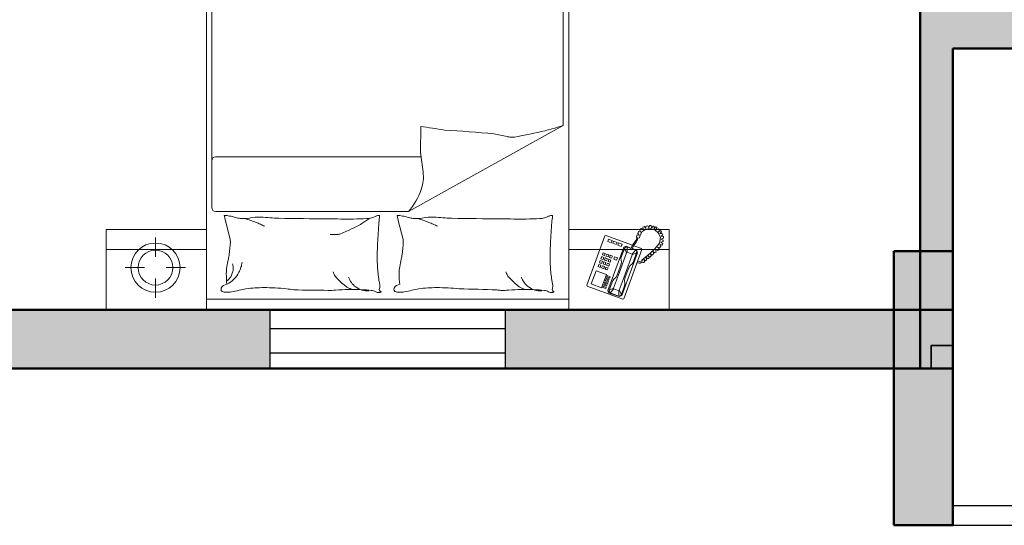
# Model space of a CAD drawing. Units: inches. Extents: x -7 to 1228, y -146 to 1091.
# Tile 21 of 88: x 664 to 815, y 36 to 113. Entities that reach past the tile are written whole.
import ezdxf

# ---------------------------------------------------------------- set-up
doc = ezdxf.new("R2010")
doc.units = ezdxf.units.IN
for name, color, linetype, lineweight in [('A-COLS', 6, 'Continuous', 35), ('A-FURN', 8, 'Continuous', 18), ('A-GLAZ', 175, 'Continuous', 25), ('A-WALL', 7, 'Continuous', 50), ('A-WALL-PATT', 251, 'Continuous', 13)]:
    doc.layers.add(name, color=color, linetype=linetype, lineweight=lineweight)
doc.styles.add('DIM_FONT', font='SIMPLEX.shx', dxfattribs={"width": 0.8})

# ---------------------------------------------------------------- blocks, each defined once
blk = doc.blocks.new('A$C4F634EDD')
for p, q in [((0, 2.6295), (0, 2.2295)), ((0.5, 2.6295), (0, 2.6295)), ((0.5, 2.6295), (2.3, 2.6295)), ((0.5, 0.5295), (0.5, 2.6295)), ((0.5, 2.2295), (0.5, 2.6295)), ((2.3, 2.6295), (2.3, 0.5295)), ((2.3, 2.6295), (2.8, 2.6295)), ((2.3, 2.2295), (2.3, 2.6295)), ((2.8, 2.6295), (2.8, 2.2295)), ((0.2457, 2.5697), (0.2457, 2.4733)), ((0.5, 2.5771), (2.3, 2.5771)), ((2.392, 2.5115), (2.5692, 2.5765)), ((2.4985, 2.5445), (2.5516, 2.564)), ((2.5062, 2.5454), (2.5004, 2.5392)), ((2.5062, 2.5454), (2.5487, 2.561)), ((2.5235, 2.5256), (2.5062, 2.5454)), ((2.5483, 2.5347), (2.5487, 2.561)), ((2.5487, 2.561), (2.5571, 2.56)), ((2.5615, 2.5536), (2.5514, 2.5318)), ((2.5516, 2.564), (2.5637, 2.5584)), ((2.5571, 2.56), (2.5615, 2.5536)), ((2.5615, 2.5536), (2.5791, 2.5058)), ((2.5637, 2.5584), (2.6418, 2.3458)), ((2.5692, 2.5765), (2.574, 2.5743)), ((2.574, 2.5743), (2.6638, 2.3298)), ((2.3898, 2.5066), (2.392, 2.5115)), ((2.4795, 2.2621), (2.3898, 2.5066)), ((2.412, 2.5007), (2.4634, 2.5196)), ((2.4361, 2.4352), (2.412, 2.5007)), ((2.4634, 2.5196), (2.4875, 2.454)), ((2.4842, 2.5232), (2.47, 2.518)), ((2.47, 2.518), (2.472, 2.5127)), ((2.472, 2.5127), (2.4862, 2.5179)), ((2.4881, 2.5126), (2.4739, 2.5074)), ((2.4739, 2.5074), (2.4759, 2.502)), ((2.4759, 2.502), (2.4901, 2.5073)), ((2.492, 2.5019), (2.4778, 2.4967)), ((2.4778, 2.4967), (2.4798, 2.4914)), ((2.4798, 2.4914), (2.494, 2.4966)), ((2.4862, 2.5179), (2.4842, 2.5232)), ((2.4901, 2.5073), (2.4881, 2.5126)), ((2.494, 2.4966), (2.492, 2.5019)), ((2.4946, 2.5331), (2.4985, 2.5445)), ((2.5734, 2.3187), (2.4946, 2.5331)), ((2.5004, 2.5392), (2.5013, 2.5315)), ((2.5013, 2.5315), (2.5188, 2.4836)), ((2.5013, 2.5315), (2.5231, 2.5214)), ((2.5231, 2.5214), (2.5235, 2.5256)), ((2.5523, 2.4417), (2.5231, 2.5214)), ((2.5483, 2.5347), (2.5235, 2.5256)), ((2.5514, 2.5318), (2.5483, 2.5347)), ((2.5807, 2.4521), (2.5514, 2.5318)), ((2.5791, 2.5058), (2.5788, 2.4956)), ((2.4875, 2.454), (2.4361, 2.4352)), ((2.4959, 2.4913), (2.4817, 2.4861)), ((2.4817, 2.4861), (2.4837, 2.4808)), ((2.4837, 2.4808), (2.4979, 2.486)), ((2.4998, 2.4807), (2.4856, 2.4755)), ((2.4856, 2.4755), (2.4876, 2.4702)), ((2.4876, 2.4702), (2.5018, 2.4754)), ((2.5037, 2.47), (2.4895, 2.4648)), ((2.4895, 2.4648), (2.4915, 2.4595)), ((2.4915, 2.4595), (2.5057, 2.4647)), ((2.4979, 2.486), (2.4959, 2.4913)), ((2.5018, 2.4754), (2.4998, 2.4807)), ((2.5057, 2.4647), (2.5037, 2.47)), ((2.5188, 2.4836), (2.5256, 2.4761)), ((2.5256, 2.4761), (2.5342, 2.4692)), ((2.5342, 2.4692), (2.5405, 2.4574)), ((2.5405, 2.4574), (2.547, 2.4397)), ((2.5788, 2.4956), (2.5767, 2.4848)), ((2.5767, 2.4848), (2.5795, 2.4717)), ((2.5795, 2.4717), (2.586, 2.454)), ((2.5807, 2.4521), (2.6158, 2.3564)), ((2.5984, 2.4204), (2.586, 2.454)), ((0.0957, 2.4197), (0.192, 2.4197)), ((0.2994, 2.4197), (0.3957, 2.4197)), ((2.4457, 2.4146), (2.4563, 2.4185)), ((2.4496, 2.4039), (2.4457, 2.4146)), ((2.4602, 2.4078), (2.4496, 2.4039)), ((2.4528, 2.3951), (2.4635, 2.399)), ((2.4563, 2.4185), (2.4602, 2.4078)), ((2.4634, 2.4211), (2.474, 2.425)), ((2.4673, 2.4104), (2.4634, 2.4211)), ((2.4635, 2.399), (2.4674, 2.3883)), ((2.4779, 2.4143), (2.4673, 2.4104)), ((2.4706, 2.4016), (2.4812, 2.4055)), ((2.4745, 2.3909), (2.4706, 2.4016)), ((2.474, 2.425), (2.4779, 2.4143)), ((2.4811, 2.4276), (2.4917, 2.4315)), ((2.485, 2.4169), (2.4811, 2.4276)), ((2.4812, 2.4055), (2.4851, 2.3949)), ((2.4956, 2.4208), (2.485, 2.4169)), ((2.4883, 2.4081), (2.4989, 2.412)), ((2.4922, 2.3975), (2.4883, 2.4081)), ((2.4917, 2.4315), (2.4956, 2.4208)), ((2.5028, 2.4014), (2.4922, 2.3975)), ((2.4989, 2.412), (2.5028, 2.4014)), ((2.5594, 2.4061), (2.547, 2.4397)), ((2.5523, 2.4417), (2.5875, 2.346)), ((2.5622, 2.393), (2.5594, 2.4061)), ((2.6047, 2.4086), (2.5984, 2.4204)), ((2.6133, 2.4017), (2.6047, 2.4086)), ((2.6201, 2.3941), (2.6133, 2.4017)), ((0.2457, 2.366), (0.2457, 2.2697)), ((2.4567, 2.3844), (2.4528, 2.3951)), ((2.4674, 2.3883), (2.4567, 2.3844)), ((2.46, 2.3756), (2.4706, 2.3795)), ((2.4639, 2.365), (2.46, 2.3756)), ((2.4745, 2.3689), (2.4639, 2.365)), ((2.4672, 2.3561), (2.4778, 2.36)), ((2.4711, 2.3455), (2.4672, 2.3561)), ((2.4706, 2.3795), (2.4745, 2.3689)), ((2.4817, 2.3494), (2.4711, 2.3455)), ((2.4851, 2.3949), (2.4745, 2.3909)), ((2.4777, 2.3821), (2.4883, 2.386)), ((2.4816, 2.3715), (2.4777, 2.3821)), ((2.4778, 2.36), (2.4817, 2.3494)), ((2.4922, 2.3754), (2.4816, 2.3715)), ((2.4849, 2.3626), (2.4955, 2.3665)), ((2.4888, 2.352), (2.4849, 2.3626)), ((2.4883, 2.386), (2.4922, 2.3754)), ((2.4994, 2.3559), (2.4888, 2.352)), ((2.4954, 2.3886), (2.5061, 2.3925)), ((2.4993, 2.378), (2.4954, 2.3886)), ((2.4955, 2.3665), (2.4994, 2.3559)), ((2.51, 2.3819), (2.4993, 2.378)), ((2.5026, 2.3691), (2.5132, 2.373)), ((2.5065, 2.3585), (2.5026, 2.3691)), ((2.5061, 2.3925), (2.51, 2.3819)), ((2.5171, 2.3624), (2.5065, 2.3585)), ((2.5132, 2.373), (2.5171, 2.3624)), ((2.5238, 2.3769), (2.538, 2.3821)), ((2.5277, 2.3663), (2.5238, 2.3769)), ((2.5419, 2.3715), (2.5277, 2.3663)), ((2.538, 2.3821), (2.5419, 2.3715)), ((2.5598, 2.372), (2.5601, 2.3822)), ((2.5774, 2.3242), (2.5598, 2.372)), ((2.5601, 2.3822), (2.5622, 2.393)), ((2.6154, 2.3522), (2.5905, 2.3431)), ((2.6158, 2.3564), (2.6154, 2.3522)), ((2.6154, 2.3522), (2.6327, 2.3324)), ((2.6376, 2.3463), (2.6158, 2.3564)), ((2.6376, 2.3463), (2.6201, 2.3941)), ((2.6499, 2.3979), (2.6397, 2.3953)), ((2.6417, 2.39), (2.6488, 2.391)), ((2.6488, 2.391), (2.6538, 2.3895)), ((2.6551, 2.397), (2.6499, 2.3979)), ((2.6538, 2.3895), (2.6596, 2.388)), ((2.6627, 2.392), (2.6551, 2.397)), ((2.6596, 2.388), (2.6626, 2.3867)), ((2.6626, 2.3867), (2.6662, 2.388)), ((2.6692, 2.394), (2.6627, 2.392)), ((2.6662, 2.388), (2.6632, 2.3828)), ((2.6632, 2.3828), (2.6736, 2.3744)), ((2.6736, 2.3944), (2.6692, 2.394)), ((2.6765, 2.391), (2.6736, 2.3944)), ((2.6736, 2.3744), (2.6922, 2.3593)), ((2.6742, 2.3795), (2.6765, 2.391)), ((2.6824, 2.3858), (2.6742, 2.3795)), ((2.6873, 2.3815), (2.6824, 2.3858)), ((2.6853, 2.369), (2.6873, 2.3815)), ((2.6946, 2.376), (2.6853, 2.369)), ((2.6922, 2.3593), (2.7051, 2.3473)), ((2.6995, 2.3713), (2.6946, 2.376)), ((2.695, 2.3603), (2.6995, 2.3713)), ((2.7031, 2.3682), (2.695, 2.3603)), ((2.7096, 2.3616), (2.7031, 2.3682)), ((2.7062, 2.351), (2.7096, 2.3616)), ((2.7147, 2.3578), (2.7062, 2.351)), ((2.7214, 2.3517), (2.7147, 2.3578)), ((2.7196, 2.34), (2.7214, 2.3517)), ((0, 2.3301), (0.5, 2.3301)), ((2.8, 2.3301), (2.3, 2.3301)), ((2.6172, 2.3086), (2.4844, 2.2599)), ((2.5362, 2.305), (2.5185, 2.2985)), ((2.5401, 2.2944), (2.5362, 2.305)), ((2.561, 2.3141), (2.5433, 2.3076)), ((2.5433, 2.3076), (2.5472, 2.297)), ((2.5472, 2.297), (2.5649, 2.3035)), ((2.5649, 2.3035), (2.561, 2.3141)), ((2.5855, 2.3131), (2.5734, 2.3187)), ((2.5774, 2.3242), (2.5875, 2.346)), ((2.5818, 2.3178), (2.5774, 2.3242)), ((2.5901, 2.3168), (2.5818, 2.3178)), ((2.6104, 2.3222), (2.5855, 2.3131)), ((2.5875, 2.346), (2.5905, 2.3431)), ((2.5905, 2.3431), (2.5901, 2.3168)), ((2.5901, 2.3168), (2.6097, 2.324)), ((2.613, 2.3312), (2.6077, 2.3293)), ((2.6077, 2.3293), (2.6135, 2.3141)), ((2.6192, 2.3174), (2.613, 2.3312)), ((2.6135, 2.3141), (2.6244, 2.2977)), ((2.6153, 2.3261), (2.6327, 2.3324)), ((2.6369, 2.332), (2.6161, 2.3243)), ((2.626, 2.3069), (2.6192, 2.3174)), ((2.6616, 2.3249), (2.6234, 2.3109)), ((2.6365, 2.2916), (2.626, 2.3069)), ((2.6327, 2.3324), (2.6385, 2.3386)), ((2.6418, 2.3458), (2.6369, 2.332)), ((2.6385, 2.3386), (2.6376, 2.3463)), ((2.6638, 2.3298), (2.6616, 2.3249)), ((2.7051, 2.3473), (2.7079, 2.3475)), ((2.7079, 2.3475), (2.7079, 2.3443)), ((2.7079, 2.3443), (2.727, 2.3277)), ((2.7286, 2.3466), (2.7196, 2.34)), ((2.727, 2.3277), (2.7512, 2.2983)), ((2.7346, 2.3423), (2.7286, 2.3466)), ((2.732, 2.3295), (2.7346, 2.3423)), ((2.7423, 2.3345), (2.732, 2.3295)), ((2.7406, 2.3172), (2.7495, 2.325)), ((2.7519, 2.3218), (2.7406, 2.3172)), ((2.7495, 2.325), (2.7423, 2.3345)), ((2.7575, 2.3144), (2.7519, 2.3218)), ((2.7526, 2.3045), (2.7575, 2.3144)), ((2.7622, 2.308), (2.7526, 2.3045)), ((2.7673, 2.2997), (2.7622, 2.308)), ((0.5953, 2.1912), (0.616, 2.2738)), ((1.4546, 2.1912), (1.4752, 2.2738)), ((2.4844, 2.2599), (2.4795, 2.2621)), ((2.5114, 2.2959), (2.4936, 2.2894)), ((2.4936, 2.2894), (2.4976, 2.2788)), ((2.4976, 2.2788), (2.5153, 2.2853)), ((2.5153, 2.2853), (2.5114, 2.2959)), ((2.5185, 2.2985), (2.5224, 2.2879)), ((2.5224, 2.2879), (2.5401, 2.2944)), ((2.6244, 2.2977), (2.6349, 2.2825)), ((2.6349, 2.2825), (2.638, 2.273)), ((2.6407, 2.2834), (2.6365, 2.2916)), ((2.6399, 2.2712), (2.6374, 2.2659)), ((2.6374, 2.2659), (2.6398, 2.257)), ((2.638, 2.273), (2.6399, 2.2712)), ((2.6398, 2.257), (2.6509, 2.259)), ((2.6438, 2.2739), (2.6407, 2.2834)), ((2.6509, 2.259), (2.6431, 2.2492)), ((2.6519, 2.2716), (2.6438, 2.2739)), ((2.6535, 2.2628), (2.6519, 2.2716)), ((2.6636, 2.2409), (2.6535, 2.2628)), ((2.756, 2.2695), (2.7459, 2.2483)), ((2.7512, 2.2983), (2.756, 2.2695)), ((2.7574, 2.2924), (2.7673, 2.2997)), ((2.7687, 2.2905), (2.7574, 2.2924)), ((2.7587, 2.279), (2.7699, 2.2828)), ((2.7708, 2.2725), (2.7587, 2.279)), ((2.759, 2.2637), (2.7706, 2.2643)), ((2.7676, 2.2559), (2.759, 2.2637)), ((2.7645, 2.2498), (2.7676, 2.2559)), ((2.7699, 2.2828), (2.7687, 2.2905)), ((2.7706, 2.2643), (2.7708, 2.2725)), ((0, 2.2295), (0.5, 2.2295)), ((2.8, 2.2295), (2.3, 2.2295)), ((2.6431, 2.2492), (2.6473, 2.2398)), ((2.6473, 2.2398), (2.6592, 2.2429)), ((2.6592, 2.2429), (2.6521, 2.2314)), ((2.6521, 2.2314), (2.6598, 2.2248)), ((2.6598, 2.2248), (2.6697, 2.2309)), ((2.6836, 2.2287), (2.6636, 2.2409)), ((2.6697, 2.2309), (2.6684, 2.219)), ((2.6684, 2.219), (2.6761, 2.2145)), ((2.6761, 2.2145), (2.6821, 2.2237)), ((2.6821, 2.2237), (2.6843, 2.2135)), ((2.7063, 2.2256), (2.6836, 2.2287)), ((2.6843, 2.2135), (2.6927, 2.2117)), ((2.6927, 2.2117), (2.6986, 2.222)), ((2.6986, 2.222), (2.7019, 2.2098)), ((2.7019, 2.2098), (2.7102, 2.2104)), ((2.7284, 2.2317), (2.7063, 2.2256)), ((2.7102, 2.2104), (2.7113, 2.2218)), ((2.7113, 2.2218), (2.7192, 2.2137)), ((2.7192, 2.2137), (2.7255, 2.2152)), ((2.7255, 2.2152), (2.7242, 2.2265)), ((2.7242, 2.2265), (2.7324, 2.2165)), ((2.7459, 2.2483), (2.7284, 2.2317)), ((2.7324, 2.2165), (2.7386, 2.2208)), ((2.7386, 2.2208), (2.7354, 2.2306)), ((2.7354, 2.2306), (2.7462, 2.2264)), ((2.7509, 2.2314), (2.7459, 2.2418)), ((2.7459, 2.2418), (2.7568, 2.2352)), ((2.7462, 2.2264), (2.7509, 2.2314)), ((2.7529, 2.2505), (2.7645, 2.2498)), ((2.7607, 2.2424), (2.7529, 2.2505)), ((2.7568, 2.2352), (2.7607, 2.2424)), ((0.5878, 2.1612), (0.5953, 2.1912)), ((1.4471, 2.1612), (1.4546, 2.1912)), ((0.5258, 2.121), (0.5258, 0.5617)), ((1.5035, 2.141), (0.5458, 2.141)), ((1.5035, 2.141), (2.2716, 1.7136)), ((1.576, 1.9433), (1.5624, 1.8479)), ((0.5458, 1.8684), (1.5653, 1.8684)), ((1.5624, 1.8479), (1.5641, 1.7178)), ((2.2716, 0.5617), (2.2716, 1.7136))]:
    blk.add_line(p, q)
for radius in [0.1222, 0.0865]:
    blk.add_circle((0.2457, 2.4197), radius)
for centre, radius, start, end in [((0.5848, 2.5274), 0.0131, 101.2724, 206.5805), ((0.6036, 2.5368), 0.0342, 206.5805, 265.5998), ((0.5999, 2.4516), 0.0904, 90, 101.2724), ((1.0898, 2.4496), 0.4918, 173.7676, 180), ((0.5999, 2.3808), 0.1611, 81.5628, 90), ((0.5368, 2.3783), 0.1399, 45.0976, 62.7964), ((0.5788, 2.2388), 0.3048, 74.256, 81.5628), ((0.7272, 2.7653), 0.2422, 254.256, 262.4531), ((0.7851, 3.2019), 0.6827, 262.4531, 270), ((0.7851, 3.5682), 1.049, 270, 276.0867), ((0.8402, 3.0514), 0.5293, 276.0867, 280.1899), ((1.1602, -8.1346), 10.6675, 90.30153, 91.21582), ((1.1169, 2.2433), 0.2897, 85.1982, 92.5386), ((1.2142, 3.4021), 0.8732, 265.1982, 269.4243), ((1.4317, 2.2032), 0.3916, 128.3886, 133.8115), ((1.2362, 2.45), 0.0768, 117.2396, 128.3886), ((1.3082, 2.3102), 0.234, 110.8603, 117.2396), ((1.2204, 4.0232), 1.4943, 269.4243, 271.9079), ((1.2995, 2.4357), 0.0992, 126.0864, 143.8234), ((1.2995, 2.4357), 0.0992, 105.9352, 126.0864), ((1.2429, 3.3501), 0.8208, 271.9079, 275.2592), ((1.2995, 2.4357), 0.0992, 85.7841, 105.9352), ((1.3132, 2.5864), 0.0539, 275.2592, 300.6513), ((1.3554, 2.5152), 0.0289, 85.6975, 120.6513), ((1.3556, 2.519), 0.0251, 68.2117, 85.6975), ((1.3739, 2.5288), 0.0156, 158.0096, 201.421), ((1.1177, 2.5413), 0.246, 347.8905, 351.8665), ((1.3634, 2.533), 0.00428, 78.1069, 158.0096), ((1.3288, 2.5111), 0.0328, 351.8665, 21.421), ((1.3647, 2.5395), 0.00232, 258.1069, 19.564), ((1.3637, 2.5391), 0.00342, 19.564, 68.2117), ((1.444, 2.5274), 0.0131, 101.2724, 206.5805), ((1.4628, 2.5368), 0.0342, 206.5805, 265.5998), ((1.4591, 2.4516), 0.0904, 90, 101.2724), ((1.949, 2.4496), 0.4918, 173.7676, 180), ((1.4591, 2.3808), 0.1611, 81.5628, 90), ((1.438, 2.2388), 0.3048, 74.256, 81.5628), ((1.5865, 2.7653), 0.2422, 254.256, 262.4531), ((1.6443, 3.2019), 0.6827, 262.4531, 270), ((1.6443, 3.5682), 1.049, 270, 276.0867), ((1.4785, 15.4878), 12.9656, 271.22425, 272.05324), ((1.97, 2.3805), 0.1524, 92.5386, 100.1899), ((1.9761, 2.2433), 0.2897, 85.1982, 92.5386), ((2.0734, 3.4021), 0.8732, 265.1982, 269.4243), ((2.291, 2.2032), 0.3916, 128.3886, 133.8115), ((2.0954, 2.45), 0.0768, 117.2396, 128.3886), ((2.1674, 2.3102), 0.234, 110.8603, 117.2396), ((2.0797, 4.0232), 1.4943, 269.4243, 271.9079), ((2.1588, 2.4357), 0.0992, 126.0864, 143.8234), ((2.1588, 2.4357), 0.0992, 105.9352, 126.0864), ((2.1021, 3.3501), 0.8208, 271.9079, 275.2592), ((2.1588, 2.4357), 0.0992, 85.7841, 105.9352), ((2.1724, 2.5864), 0.0539, 275.2592, 300.6513), ((2.2146, 2.5152), 0.0289, 85.6975, 120.6513), ((2.2149, 2.519), 0.0251, 68.2117, 85.6975), ((2.2331, 2.5288), 0.0156, 158.0096, 201.421), ((1.977, 2.5413), 0.246, 347.8905, 351.8665), ((2.2226, 2.533), 0.00428, 78.1069, 158.0096), ((2.1881, 2.5111), 0.0328, 351.8665, 21.421), ((2.224, 2.5395), 0.00232, 258.1069, 19.564), ((2.2229, 2.5391), 0.00342, 19.564, 68.2117), ((0.8019, 2.4496), 0.204, 180, 189.6844), ((0.5462, 2.4142), 0.0899, 41.4429, 53.7359), ((0.5741, 2.4389), 0.0526, 25.3551, 41.4429), ((0.4851, 2.3967), 0.1511, 21.8149, 25.3551), ((0.4345, 2.3765), 0.2056, 18.7799, 21.8149), ((0.5368, 2.3783), 0.1399, 27.3988, 45.0976), ((1.3127, 2.3625), 0.2002, 151.6832, 156.9972), ((1.1799, 2.4341), 0.0493, 140.9651, 151.6832), ((1.3165, 2.3233), 0.2252, 133.8115, 140.9651), ((1.2995, 2.4357), 0.0992, 143.8234, 161.5603), ((2.2605, 2.3525), 0.9131, 172.3191, 176.6313), ((1.5522, 2.448), 0.1983, 167.8905, 172.3191), ((1.6611, 2.4496), 0.204, 180, 189.6844), ((2.1719, 2.3625), 0.2002, 151.6832, 156.9972), ((2.0391, 2.4341), 0.0493, 140.9651, 151.6832), ((2.1757, 2.3233), 0.2252, 133.8115, 140.9651), ((2.1588, 2.4357), 0.0992, 143.8234, 161.5603), ((3.1198, 2.3525), 0.9131, 172.3191, 176.6313), ((2.4114, 2.448), 0.1983, 167.8905, 172.3191), ((1.4703, 2.5637), 0.882, 189.6844, 192.1984), ((0.576, 2.4246), 0.0562, 0, 18.7799), ((0.5406, 2.4246), 0.0915, 345.3149, 0), ((0.5368, 2.3783), 0.1399, 16.515, 27.3988), ((0.5368, 2.3783), 0.1399, 5.6311, 16.515), ((2.0266, 2.3663), 0.6787, 176.6313, 181.6331), ((2.3295, 2.5637), 0.882, 189.6844, 192.1984), ((2.8858, 2.3663), 0.6787, 176.6313, 181.6331), ((0.2982, 2.3103), 0.3171, 8.0051, 12.1984), ((-0.0401, 2.2627), 0.6588, 2.6649, 8.0051), ((1.1575, 2.3103), 0.3171, 8.0051, 12.1984), ((0.8191, 2.2627), 0.6588, 2.6649, 8.0051), ((2.7128, 2.3859), 1.3652, 181.6331, 183.055), ((14.9657, 3.0398), 13.6356, 183.05496, 183.50486), ((3.5721, 2.3859), 1.3652, 181.6331, 183.055), ((15.8249, 3.0398), 13.6356, 183.05496, 183.50486), ((0.5503, 2.2902), 0.0677, 345.9548, 2.6649), ((1.1303, 1.9835), 0.2721, 85.9172, 93.5552), ((1.1455, 2.197), 0.058, 69.3257, 85.9172), ((1.4096, 2.2902), 0.0677, 345.9548, 2.6649), ((0.473, 2.8815), 0.7387, 291.6577, 293.4844), ((0.473, 2.8815), 0.7387, 293.4844, 295.3111), ((0.9871, 1.7772), 0.5066, 65.6735, 69.3257), ((0.6058, 0.9338), 1.4323, 63.5015, 65.6735), ((1.1054, 1.9358), 0.3126, 57.865, 63.5015), ((1.6762, 2.2258), 0.3212, 183.5049, 189.9984), ((1.3322, 2.8815), 0.7387, 291.6577, 293.4844), ((1.3322, 2.8815), 0.7387, 293.4844, 295.3111), ((2.5355, 2.2258), 0.3212, 183.5049, 189.9984), ((0.5887, 2.1609), 0.000917, 165.9551, 274.0829), ((0.5695, 2.4301), 0.2708, 274.0829, 279.4841), ((0.5763, 2.3896), 0.2297, 279.4841, 287.3864), ((0.6807, 2.0561), 0.1197, 96.4341, 107.3864), ((0.6836, 2.0301), 0.1459, 78.4414, 96.4341), ((0.473, 2.8815), 0.7387, 287.1982, 289.428), ((0.759, 2.3985), 0.2301, 258.4414, 272.7491), ((0.473, 2.8815), 0.7387, 289.428, 291.6577), ((0.7026, 3.5718), 1.4048, 272.7491, 274.6176), ((0.9136, 0.9591), 1.2165, 92.6096, 94.6176), ((1.2501, -19.8405), 22.0183, 90.37908, 91.01965), ((1.2012, -3.5404), 5.7185, 89.7135, 90.9704), ((1.224, 1.0141), 1.164, 86.426, 89.7135), ((0.8841, 1.5835), 0.7286, 54.1737, 57.865), ((1.2875, 2.0302), 0.1459, 77.131, 86.426), ((1.3099, 2.1283), 0.0453, 62.7159, 77.131), ((1.3658, 2.2367), 0.0767, 242.7159, 253.7788), ((1.3688, 2.247), 0.0875, 253.7788, 262.8796), ((1.3581, 2.1615), 0.00132, 262.8796, 343.3022), ((1.3409, 2.1667), 0.0193, 343.3022, 9.9984), ((1.448, 2.1609), 0.000917, 165.9551, 274.0829), ((1.4288, 2.4301), 0.2708, 274.0829, 279.4841), ((1.4355, 2.3896), 0.2297, 279.4841, 287.3864), ((1.5399, 2.0561), 0.1197, 96.4341, 107.3864), ((1.5429, 2.0301), 0.1459, 78.4414, 96.4341), ((1.3322, 2.8815), 0.7387, 287.1982, 289.428), ((1.6182, 2.3985), 0.2301, 258.4414, 272.7491), ((1.3322, 2.8815), 0.7387, 289.428, 291.6577), ((1.5619, 3.5718), 1.4048, 272.7491, 274.6176), ((1.7729, 0.9591), 1.2165, 92.6096, 94.6176), ((2.1093, -19.8405), 22.0183, 90.37908, 91.01965), ((2.0605, -3.5404), 5.7185, 89.7135, 90.9704), ((2.0833, 1.0141), 1.164, 86.426, 89.7135), ((2.1467, 2.0302), 0.1459, 77.131, 86.426), ((2.1691, 2.1283), 0.0453, 62.7159, 77.131), ((2.2251, 2.2367), 0.0767, 242.7159, 253.7788), ((2.2281, 2.247), 0.0875, 253.7788, 262.8796), ((2.2174, 2.1615), 0.00132, 262.8796, 343.3022), ((2.2001, 2.1667), 0.0193, 343.3022, 9.9984), ((0.5458, 2.121), 0.02, 90, 180), ((1.2147, 1.9017), 0.3751, 20.1488, 39.6445), ((1.3977, 1.9688), 0.1801, 351.8644, 20.1488), ((0.5458, 1.8884), 0.02, 180, 270), ((1.4194, 4.2174), 2.5158, 281.6741, 283.1904), ((2.0378, 1.5789), 0.1942, 97.7304, 103.1904), ((2.0195, 1.7137), 0.0581, 79.2724, 97.7304), ((1.2737, -2.2227), 4.0646, 77.0745, 79.2724), ((1.0582, 5.4638), 3.7801, 277.692, 279.495), ((0.6102, 18.0525), 16.3521, 273.75703, 274.62393), ((2.0359, 1.0981), 0.6574, 74.0648, 77.0745), ((1.7125, -0.0344), 1.8351, 72.2636, 74.0648)]:
    blk.add_arc(centre, radius, start, end)
at = {"style": 'DIM_FONT', "width": 0.8, "flags": 9}
for tag, p in [('YSIZE', (0.5, 2.6295)), ('XSIZE', (0.5, 2.6295)), ('XSIZE', (2.2985, 2.6295)), ('YSIZE', (2.2985, 2.6295))]:
    blk.add_attdef(tag, p, '', height=0.0005, dxfattribs=at)
blk = doc.blocks.new('WIN-36')
for p, q in [((0, 36), (0, 0)), ((9, 36), (0, 36)), ((2.34, 36), (2.34, 0)), ((6.14, 0), (6.14, 36)), ((9, 0), (9, 36)), ((0, 0), (9, 0)), ((2.34, 0), (6.14, 0))]:
    blk.add_line(p, q)

msp = doc.modelspace()

# ---------------------------------------------------------------- hatches: boundary and pattern name
at = {"layer": 'A-COLS'}
h = msp.add_hatch(color=256, dxfattribs=at)
h.dxf.hatch_style = 1
h.paths.add_polyline_path([(807, 78), (798, 78), (798, 60), (803.71, 60), (803.71, 63.55), (807, 63.55)])
h = msp.add_hatch(color=256, dxfattribs=at)
h.dxf.hatch_style = 1
h.paths.add_polyline_path([(803.71, 63.55), (803.71, 60), (807, 60), (807, 63.55)])
at = {"layer": 'A-WALL-PATT'}
h = msp.add_hatch(color=256, dxfattribs=at)
h.dxf.hatch_style = 1
h.paths.add_polyline_path([(69, 568), (60, 568), (60, 493), (63.29, 493), (69, 493)])
h.paths.add_polyline_path([(69, 662.41), (60, 662.41), (60, 586), (69, 586)], flags=17)
h.paths.add_polyline_path([(69, 723), (184, 723), (184, 734), (179, 734), (179, 728), (69, 728), (69, 741.62), (60, 741.62), (60, 698.41), (69, 698.41)], flags=17)
h.paths.add_polyline_path([(69, 782), (231, 782), (231, 728), (231, 723), (231, 586), (236, 586), (236, 787), (69, 787), (69, 800.13), (60, 800.13), (60, 765.62), (69, 765.62)])
h.paths.add_polyline_path([(184, 842), (189, 842), (189, 848), (173, 848), (173, 842), (179, 842), (179, 787), (184, 787)])
h.paths.add_polyline_path([(118.22, 69), (69, 69), (69, 60), (118.22, 60)])
h.paths.add_polyline_path([(227, 69), (154.22, 69), (154.22, 60), (227, 60)])
h.paths.add_polyline_path([(236, 60), (232.71, 60), (227, 60), (227, 36), (236, 36)])
h.paths.add_polyline_path([(389, 60), (380, 60), (380, 36), (389, 36)])
h.paths.add_polyline_path([(384, 181), (380, 181), (380, 115), (380, 78), (384, 78)])
h.paths.add_polyline_path([(380, 115), (334.55, 115), (334.55, 109), (380, 109)])
h.paths.add_polyline_path([(274.55, 115), (236, 115), (236, 201), (232.71, 201), (231, 201), (231, 78), (236, 78), (236, 109), (274.55, 109)])
h.paths.add_polyline_path([(69, 123), (60, 123), (60, 78), (69, 78)])
h.paths.add_polyline_path([(69, 201), (60, 201), (60, 159), (69, 159)])
h.paths.add_polyline_path([(143, 219), (69, 219), (69, 213), (143, 213)], flags=17)
h.paths.add_polyline_path([(189, 219), (184, 219), (184, 274), (231, 274), (231, 219), (236, 219), (236, 279), (184, 279), (184, 297), (179, 297), (179, 279), (69, 279), (69, 290.91), (60, 290.91), (60, 262.18), (69, 262.18), (69, 274), (179, 274), (179, 219), (173, 219), (173, 213), (189, 213)])
h.paths.add_polyline_path([(69, 238.18), (60, 238.18), (60, 219), (69, 219)], flags=17)
h.paths.add_polyline_path([(69, 333), (60, 333), (60, 314.91), (69, 314.91), (69, 316.96)])
h.paths.add_polyline_path([(190, 338), (184, 338), (69, 338), (69, 333), (179, 333), (179, 327), (184, 327), (184, 333.02), (190, 333.05)])
h.paths.add_polyline_path([(69, 386.81), (60, 386.81), (60, 351), (69, 351)])
h.paths.add_polyline_path([(69, 475), (60, 475), (60, 422.81), (69, 422.81)])
h.paths.add_polyline_path([(236, 475), (231, 475), (231, 351.24), (236, 351.24)])
h.paths.add_polyline_path([(384, 475), (380, 475), (380, 362), (384, 362)])
h.paths.add_polyline_path([(547, 307), (439, 307), (439, 356), (445, 356), (445, 362), (433, 362), (433, 307), (380, 307), (380, 244), (380, 241), (384, 241), (384, 301), (433, 301), (433, 277), (439, 277), (439, 301), (547, 301)])
h.paths.add_polyline_path([(547, 241), (439, 241), (439, 247), (433, 247), (433, 235), (547, 235)])
h.paths.add_polyline_path([(450, 69), (440.29, 69), (424.89, 69), (389, 69), (389, 60), (450, 60)])
h.paths.add_polyline_path([(547, 69), (486, 69), (486, 60), (547, 60)])
h.paths.add_polyline_path([(556, 148.27), (547, 148.27), (547, 78), (556, 78)])
h.paths.add_polyline_path([(556, 223), (547, 223), (547, 195), (547, 184.27), (556, 184.27)])
h.paths.add_polyline_path([(556, 311.19), (547, 311.19), (547, 273.08), (556, 273.08)])
h.paths.add_polyline_path([(556, 344), (552.71, 344), (547, 344), (547, 335.19), (556, 335.19)])
h.paths.add_polyline_path([(556, 249.08), (547, 249.08), (547, 241), (556, 241)])
h.paths.add_polyline_path([(547, 362), (475, 362), (475, 356), (547, 356)], flags=0)
h.paths.add_polyline_path([(556, 399.62), (547, 399.62), (547, 362), (556, 362)])
h.paths.add_polyline_path([(556, 475), (547, 475), (547, 435.62), (556, 435.62)])
h.paths.add_polyline_path([(547, 493), (389, 493), (389, 487), (547, 487)])
h.paths.add_polyline_path([(380, 493), (278, 493), (278, 487), (380, 487)])
h.paths.add_polyline_path([(227, 493), (69, 493), (69, 487), (227, 487)])
h.paths.add_polyline_path([(643, 122.44), (634, 122.44), (634, 78), (643, 78)])
h.paths.add_polyline_path([(702.5, 69), (692.79, 69), (677.39, 69), (643, 69), (643, 60), (702.5, 60)])
h.paths.add_polyline_path([(798, 69), (738.5, 69), (738.5, 60), (798, 60)])
h.paths.add_polyline_path([(807, 60), (803.71, 60), (798, 60), (798, 36), (807, 36)])
h.paths.add_polyline_path([(807, 109), (846.75, 109), (846.75, 115), (807, 115), (807, 159), (802, 159), (802, 78), (807, 78)])
h.paths.add_polyline_path([(807, 201), (802, 201), (802, 195), (807, 195)])
h.paths.add_polyline_path([(643, 201), (634, 201), (634, 158.44), (643, 158.44)])
h.paths.add_polyline_path([(756, 225), (751, 225), (751, 219), (643, 219), (643, 213), (756, 213)])
h.paths.add_polyline_path([(643, 240.85), (634, 240.85), (634, 219), (643, 219)])
h.paths.add_polyline_path([(643, 274), (643, 288.63), (634, 288.63), (634, 264.85), (643, 264.85)])
h.paths.add_polyline_path([(802, 279), (756, 279), (756, 297), (751, 297), (751, 279), (643, 279), (643, 274), (751, 274), (751, 255), (756, 255), (756, 274), (802, 274)])
h.paths.add_polyline_path([(807, 333), (803.71, 333), (802, 333), (802, 279), (802, 274), (802, 219), (807, 219)])
h.paths.add_polyline_path([(956, 182), (951, 182), (951, 115), (906.75, 115), (906.75, 109), (951, 109), (951, 78), (956, 78)])
h.paths.add_polyline_path([(960, 60), (951, 60), (951, 36), (960, 36)])
h.paths.add_polyline_path([(1021, 69), (1005.78, 69), (960, 69), (960, 60), (1021, 60)])
h.paths.add_polyline_path([(956, 224), (951, 224), (951, 218), (956, 218)])
h.paths.add_polyline_path([(956, 302), (1004, 302), (1004, 278), (1010, 278), (1010, 302), (1118, 302), (1118, 290.81), (1127, 290.81), (1127, 326.97), (1118, 326.97), (1118, 320.97), (1118, 307), (1010, 307), (1010, 356), (1016, 356), (1016, 362), (1004, 362), (1004, 307), (951, 307), (951, 244), (951, 242), (954.29, 242), (956, 242)])
h.paths.add_polyline_path([(643, 333), (634, 333), (634, 312.63), (643, 312.63), (643, 316.96)])
h.paths.add_polyline_path([(756, 338), (643, 338), (643, 333), (751, 333), (751, 327), (756, 327)])
h.paths.add_polyline_path([(643, 388), (634, 388), (634, 351), (643, 351)])
h.paths.add_polyline_path([(807, 357), (802, 357), (802, 351), (807, 351)])
h.paths.add_polyline_path([(807, 475), (802, 475), (802, 393), (807, 393)])
h.paths.add_polyline_path([(643, 475), (634, 475), (634, 424), (643, 424)])
h.paths.add_polyline_path([(798, 493), (643, 493), (643, 487), (798, 487)])
h.paths.add_polyline_path([(634, 493), (556, 493), (556, 487), (634, 487)])
h.paths.add_polyline_path([(813, 493), (807, 493), (807, 487), (813, 487)])
h.paths.add_polyline_path([(951, 493), (849, 493), (849, 487), (951, 487)])
h.paths.add_polyline_path([(956, 484), (951, 484), (951, 374), (956, 374)])
h.paths.add_polyline_path([(1109, 493), (969, 493), (969, 487), (1109, 487)])
h.paths.add_polyline_path([(1127, 484), (1118, 484), (1118, 450.64), (1127, 450.64)])
h.paths.add_polyline_path([(1127, 414.64), (1118, 414.64), (1118, 365), (1127, 365)])
h.paths.add_polyline_path([(1109, 362), (1046, 362), (1046, 356), (1109, 356)], flags=17)
h.paths.add_polyline_path([(1127, 356), (1123.45, 356), (1118, 356), (1118, 350.97), (1127, 350.97)], flags=0)
h.paths.add_polyline_path([(1127, 266.81), (1118, 266.81), (1118, 262.36), (1118, 242), (1127, 242)], flags=17)
h.paths.add_polyline_path([(1118, 242), (1010, 242), (1010, 248), (1004, 248), (1004, 237), (1118, 237)])
h.paths.add_polyline_path([(1127, 224), (1118, 224), (1118, 170), (1127, 170)])
h.paths.add_polyline_path([(1127, 134), (1118, 134), (1118, 78), (1127, 78)])
h.paths.add_polyline_path([(1118, 69), (1057, 69), (1057, 60), (1118, 60)])
h.paths.add_polyline_path([(227, 571.55), (227, 574), (69, 574), (69, 568), (227, 568)])
h.paths.add_polyline_path([(380, 571.55), (380, 574), (278, 574), (278, 568), (380, 568)])
h.paths.add_polyline_path([(242, 574), (236, 574), (236, 568), (242, 568)])
h.paths.add_polyline_path([(547, 571.55), (547, 574), (389, 574), (389, 568), (547, 568)])
h.paths.add_polyline_path([(384, 733), (380, 733), (380, 586), (384, 586)])
h.paths.add_polyline_path([(556, 646), (634, 646), (634, 655), (547, 655), (547, 586), (556, 586)])
h.paths.add_polyline_path([(634, 574), (556, 574), (556, 568), (634, 568)])
h.paths.add_polyline_path([(643, 655), (634, 655), (634, 586), (643, 586)])
h.paths.add_polyline_path([(798, 574), (643, 574), (643, 568), (798, 568)])
h.paths.add_polyline_path([(643, 663.85), (634, 663.85), (634, 655), (643, 655)])
h.paths.add_polyline_path([(556, 676.97), (547, 676.97), (547, 655), (556, 655)])
h.paths.add_polyline_path([(556, 733), (547, 733), (547, 712.97), (556, 712.97)])
h.paths.add_polyline_path([(643, 710), (634, 710), (634, 699.85), (643, 699.85)])
h.paths.add_polyline_path([(807, 668), (802, 668), (802, 586), (807, 586)])
h.paths.add_polyline_path([(951, 574), (849, 574), (849, 568), (951, 568)])
h.paths.add_polyline_path([(956, 691), (951, 691), (951, 577), (956, 577)])
h.paths.add_polyline_path([(1109, 574), (969, 574), (969, 568), (1109, 568)])
h.paths.add_polyline_path([(1127, 643.4), (1118, 643.4), (1118, 577), (1127, 577)])
h.paths.add_polyline_path([(1127, 568), (1123.45, 568), (1118, 568), (1118, 493), (1127, 493)])
h.paths.add_polyline_path([(1127, 733), (1118, 733), (1118, 679.4), (1127, 679.4)])
h.paths.add_polyline_path([(1127, 777.35), (1118, 777.35), (1118, 770.04), (1118, 751), (1127, 751)], flags=17)
h.paths.add_polyline_path([(1118, 751), (1010, 751), (1010, 757), (1004, 757), (1004, 745), (1118, 745)])
h.paths.add_polyline_path([(956, 811), (1004, 811), (1004, 787), (1010, 787), (1010, 811), (1017.87, 811), (1017.87, 811.63, -0.414214), (1018.25, 812), (1031.98, 812, -0.414214), (1032.35, 811.63), (1032.35, 811), (1118, 811), (1118, 801.35), (1127, 801.35), (1127, 834.69), (1118, 834.69), (1118, 830.24), (1118, 817), (1010, 817), (1010, 866), (1016, 866), (1016, 872), (1004, 872), (1004, 817), (956, 817), (956, 866), (951, 866), (951, 751), (954.29, 751), (956, 751)])
h.paths.add_polyline_path([(1118, 872), (1046, 872), (1046, 866), (1118, 866)], flags=17)
h.paths.add_polyline_path([(1127, 924.71), (1118, 924.71), (1118, 884), (1127, 884)])
h.paths.add_polyline_path([(1127, 866), (1123.71, 866), (1118, 866), (1118, 858.69), (1127, 858.69)], flags=17)
h.paths.add_polyline_path([(956, 983), (951, 983), (951, 952), (807, 952), (807, 983), (802, 983), (802, 902), (807, 902), (807, 946), (951, 946), (951, 884), (956, 884)])
h.paths.add_polyline_path([(807, 842), (802, 842), (802, 787), (756, 787), (756, 806), (751, 806), (751, 787), (643, 787), (643, 782), (751, 782), (751, 764), (756, 764), (756, 782), (802, 782), (802, 728), (807, 728)])
h.paths.add_polyline_path([(756, 848), (643, 848), (643, 842), (751, 842), (751, 836), (756, 836)])
h.paths.add_polyline_path([(756, 734), (751, 734), (751, 728), (643, 728), (643, 723), (756, 723)])
h.paths.add_polyline_path([(643, 749.79), (634, 749.79), (634, 728), (637.29, 728), (643, 728)])
h.paths.add_polyline_path([(643, 805.41), (634, 805.41), (634, 773.79), (643, 773.79)])
h.paths.add_polyline_path([(643, 896.66), (634, 896.66), (634, 860), (637.29, 860), (643, 860)])
h.paths.add_polyline_path([(643, 842), (634, 842), (634, 829.41), (643, 829.41)])
h.paths.add_polyline_path([(643, 983), (634, 983), (634, 932.66), (643, 932.66)])
h.paths.add_polyline_path([(1127, 983), (1118, 983), (1118, 960.71), (1127, 960.71)])
h.paths.add_polyline_path([(1118, 1001), (1077.53, 1001), (1077.53, 992), (1118, 992)])
h.paths.add_polyline_path([(1041.53, 1001), (960, 1001), (960, 992), (1041.53, 992)])
h.paths.add_polyline_path([(960, 1025), (951, 1025), (951, 1001), (954.29, 1001), (960, 1001)])
h.paths.add_polyline_path([(807, 1025), (798, 1025), (798, 1001), (807, 1001)])
h.paths.add_polyline_path([(798, 1001), (738.5, 1001), (738.5, 992), (798, 992)])
h.paths.add_polyline_path([(702.5, 1001), (643, 1001), (643, 992), (702.5, 992)])
h.paths.add_polyline_path([(547, 1001), (499.11, 1001), (499.11, 992), (547, 992)])
h.paths.add_polyline_path([(463.11, 1001), (389, 1001), (389, 992), (463.11, 992)])
h.paths.add_polyline_path([(389, 1025), (380, 1025), (380, 1022), (380, 1001), (383.29, 1001), (389, 1001)])
h.paths.add_polyline_path([(236, 1025), (227, 1025), (227, 1001), (236, 1001)])
h.paths.add_polyline_path([(236, 983), (231, 983), (231, 860), (236, 860)])
h.paths.add_polyline_path([(274.55, 952), (236, 952), (236, 946), (274.55, 946)])
h.paths.add_polyline_path([(380, 952), (334.55, 952), (334.55, 946), (380, 946)])
h.paths.add_polyline_path([(384, 983), (380, 983), (380, 884), (383.29, 884), (384, 884)])
h.paths.add_polyline_path([(227, 1001), (155.01, 1001), (155.01, 992), (162.87, 992), (227, 992)])
h.paths.add_polyline_path([(119.01, 1001), (69, 1001), (69, 992), (119.01, 992)])
h.paths.add_polyline_path([(69, 983), (60, 983), (60, 922.99), (69, 922.99)])
h.paths.add_polyline_path([(69, 886.99), (60, 886.99), (60, 860), (63.29, 860), (69, 860)])
h.paths.add_polyline_path([(143, 848), (69, 848), (69, 842), (143, 842)])

# ---------------------------------------------------------------- linework, layer by layer
at = {"layer": 'A-COLS'}
msp.add_lwpolyline([(807, 60), (803.71, 60), (803.71, 63.55), (807, 63.55)], close=True, dxfattribs=at)
at = {"layer": 'A-GLAZ'}
for p, q in [((951, 39), (807, 39)), ((807, 36), (951, 36))]:
    msp.add_line(p, q, dxfattribs=at)
at = {"layer": 'A-WALL'}
for p, q in [((802, 159.35), (802, 60)), ((802, 60), (802, 159)), ((807, 60), (807, 109)), ((951, 109), (807, 109)), ((807, 109), (807, 60)), ((798, 60), (798, 78)), ((798, 78), (807, 78)), ((807, 78), (807, 60)), ((807, 69), (634, 69)), ((380, 60), (807, 60)), ((807, 60), (634, 60)), ((807, 60), (798, 60)), ((798, 60), (798, 36)), ((807, 36), (807, 60)), ((798, 36), (807, 36))]:
    msp.add_line(p, q, dxfattribs=at)

# ---------------------------------------------------------------- block references
at = {"layer": 'A-FURN', "xscale": -30.79356024027943, "yscale": 30.79356024027943, "zscale": 30.79356024027943, "rotation": 180}
msp.add_blockref('A$C4F634EDD', (677.39, 149.97), dxfattribs=at)
at = {"layer": 'A-GLAZ', "extrusion": (0, 0, -1), "zscale": -1, "rotation": 90.00000000000003}
msp.add_blockref('WIN-36', (-702.5, 60), dxfattribs=at)

doc.saveas('drawing.dxf')
